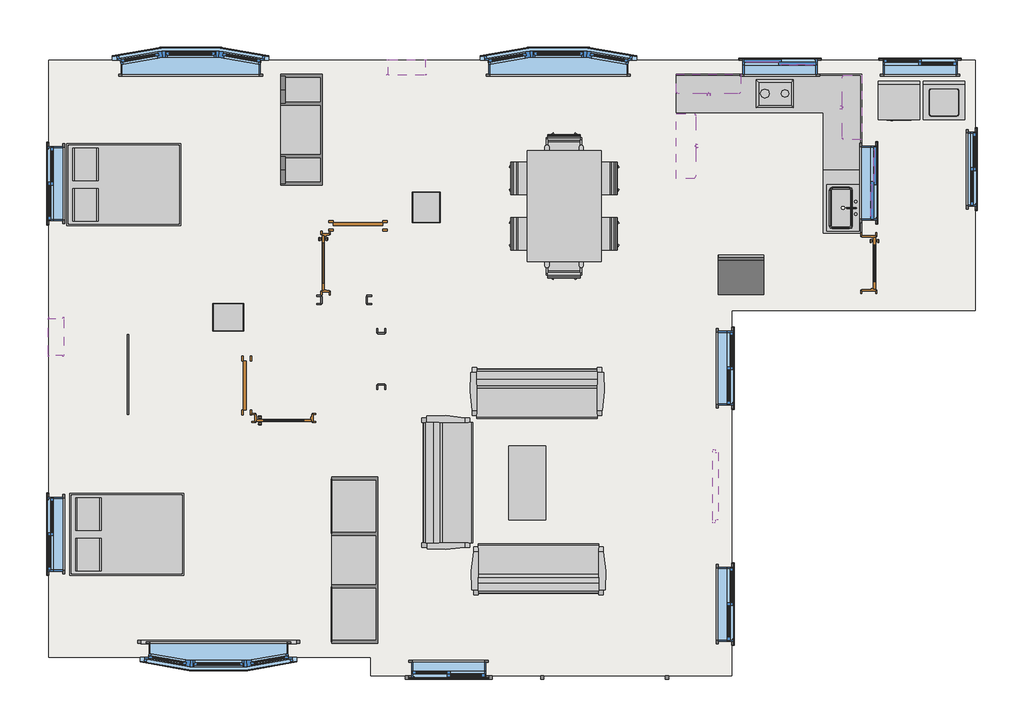
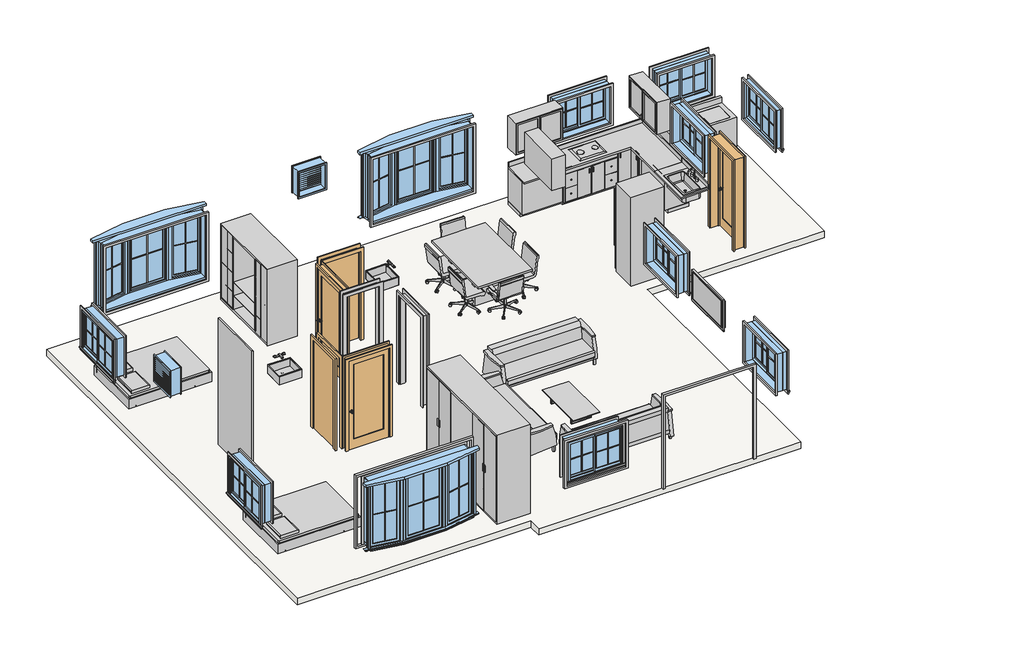
# One storey, incomplete: 54 proxies, 27 furniture elements, 14 windows, 5 doors, 3 flow terminals, 1 plate, 1 slab.
# Revit data of these elements (continued)
# Type "Window-Bay-Casement-10_Degree_Angle : 90\" x 60\" x 6\"" (continued)
#   Exterior Trim = element 406593
#   Interior Trim = Trim-Window-Interior-Flat : Picture Frame
#   Interior Frame Material = Wood - Stained
#   Glass Panel Material = Glass
#   Exterior Frame Material = Clad - White
#   Wall Closure = (empty or 0)
# Type "Window-Louvers : 24\" x 24\""
#   Type Mark = "21"
#   Construction Type Id = "GSP4R"
#   Assembly Code = "B20"
#   Analytic Construction = "1/8 in Pilkington single glazing"
#   Visual Light Transmittance = 0.9
#   Thermal Resistance (R) = 1.53941 (h·ft²·°F)/BTU
#   Solar Heat Gain Coefficient = 0.78
#   Max Height = 1' - 11.74264"
#   Height = 2' - 0"
#   Heat Transfer Coefficient (U) = 0.6496 BTU/(h·ft²·°F)
#   Blade Width [instance default] = 1' - 10 1/2"
#   Blade Vertical Thickness = 0' - 0.35355"
#   Blade Thickness = 0' - 0 1/4"
#   Blade Spacing = 0' - 1 1/2"
#   Blade Height = 0' - 1.85355"
#   Blade Depth = 0' - 3"
#   Blade Angle = 45.00°
#   Default Sill Height = 3' - 0"
#   Trim Projection_Exterior = 0' - 0 1/2"
#   Trim Projection_Interior = 0' - 0 1/2"
#   Trim Width_Exterior = 0' - 1 1/2"
#   Trim Width_Interior = 0' - 1 1/2"
#   Width = 2' - 0"
#   Max Blade Count = 12
#   Define Thermal Properties by = 1
#   Blade Count = 12
#   Frame Material = Birch
#   Louver Material = Birch
#   Trim Exterior Material = Birch
#   Trim Interior Material = Birch
#   Wall Closure = (empty or 0)
# Type "Window-Sliding-Double : 48\" x 36\""
#   Type Mark = "20"
#   Fire Rating = "0.5h"
#   Assembly Code = "B2020100"
#   Analytic Construction = "Double glazing - domestic"
#   Window Inset [instance default] = 0' - 0"
#   Wall Thickness [instance default] = 0' - 6"
#   Visual Light Transmittance = 0.81
#   Thermal Resistance (R) = 1.8146 (h·ft²·°F)/BTU
#   Solar Heat Gain Coefficient = 0.76
#   Muntin Width = 1' - 8 5/8"
#   Muntin Height = 2' - 6 1/4"
#   Interior Wall Closure [instance default] = 0' - 2 3/4"
#   Heat Transfer Coefficient (U) = 0.5511 BTU/(h·ft²·°F)
#   Frame Extension [instance default] = 0' - 0 1/4"
#   Exterior Wall Closure [instance default] = 0' - 1 1/4"
#   Rough Width = 4' - 0 1/2"
#   Rough Height = 3' - 0 1/2"
#   Height = 3' - 0"
#   Extension Jamb [instance default] = 0' - 2 3/4"
#   Default Sill Height = 3' - 0"
#   Width = 4' - 0"
#   Interior Trim Visibility [instance default] = yes
#   Indicator Visibility [instance default] = yes
#   Exterior Trim Visibility [instance default] = yes
#   Muntin Visibility = yes
#   Extension Jamb Visibility [instance default] = yes
#   Muntin Pattern = Muntin Pattern_2x2 : Muntin Pattern_2x2
#   Interior Trim Material = Wood - Stained
#   Interior Trim = Trim-Window-Interior-Flat : Picture Frame
#   Interior Frame Material = Wood - Stained
#   Glass Panel Material = Glass
#   Exterior Trim Material = Clad - White
#   Exterior Trim = Trim-Window-Exterior-Flat : with Sill
#   Exterior Frame Material = Clad - White
#   Wall Closure = (empty or 0)
# Element 1 (IfcBuildingElementProxy, "Cook Top-2 Unit : 12\" x 18\" 2")
#   Phase Created = New Construction
#   Materials on its faces: "Metal - Steel, Polished", "Metal - Chrome"
# Element 2 (IfcBuildingElementProxy, "Dryer : 27\" x 25\" x 35\"")
#   Phase Created = New Construction
#   Materials on its faces: "Metal - Paint Finish - Ivory,Glossy"
# Elements 3, 4, 5 (IfcBuildingElementProxy, "Muntin Pattern_2x2 : Muntin Pattern_2x2")
#   Width = 2' - 3.57789"
#   Height = 4' - 6 1/2"
#   Interior Material = Wood - Stained
#   Exterior Material = Clad - White
#   Phase Created = New Construction
#   Materials on its faces: "Clad - White", "Wood - Stained"
# Elements 6, 7, 8, 9, 10, 11 (IfcBuildingElementProxy, "Muntin Pattern_2x2 : Muntin Pattern_2x2")
#   Width = 1' - 7.85416"
#   Height = 4' - 6 1/2"
#   Interior Material = Wood - Stained
#   Exterior Material = Clad - White
#   Phase Created = New Construction
#   Materials on its faces: "Clad - White", "Wood - Stained"
# Elements 12, 13, 14, 15, 16, 17, 18, 19, 20, 21, 22, 23, 24, 25, 26, 27, 28, 29 (IfcBuildingElementProxy, "Muntin Pattern_2x2 : Muntin Pattern_2x2")
#   Width = 1' - 8 5/8"
#   Height = 2' - 6 1/4"
#   Interior Material = Wood - Stained
#   Exterior Material = Clad - White
#   Phase Created = New Construction
#   Materials on its faces: "Clad - White", "Wood - Stained"
# Element 30 (IfcBuildingElementProxy, "Passage Opening-Cased : 30\" x 84\"")
#   Phase Created = New Construction
#   Materials on its faces: "Door - Frame"
# Element 31 (IfcBuildingElementProxy, "Passage Opening-Cased : 34\" x 84\"")
#   Phase Created = New Construction
#   Materials on its faces: "Door - Frame"
# Element 32 (IfcBuildingElementProxy, "Refrigerator-Built-in : 30\" x 24\" LH")
#   Phase Created = New Construction
#   Materials on its faces: "Metal - Paint Finish - Ivory,Glossy", "Metal - Chrome"
# Elements 33, 34, 35, 36, 37, 38, 39, 40, 41 (IfcBuildingElementProxy, "Trim-Window-Exterior-Flat : with Sill")
#   Opening Width = 4' - 0"
#   Opening Height = 3' - 0"
#   Trim Material = Clad - White
#   Phase Created = New Construction
#   Materials on its faces: "Clad - White"
# Elements 42, 43, 44 (IfcBuildingElementProxy, "Trim-Window-Interior-Flat : Picture Frame")
#   Opening Width = 7' - 6"
#   Opening Height = 5' - 2"
#   Trim Material = Wood - Stained
#   Phase Created = New Construction
#   Materials on its faces: "Wood - Stained"
# Elements 45, 46, 47, 48, 49, 50, 51, 52, 53 (IfcBuildingElementProxy, "Trim-Window-Interior-Flat : Picture Frame")
#   Opening Width = 4' - 0"
#   Opening Height = 3' - 0"
#   Trim Material = Wood - Stained
#   Phase Created = New Construction
#   Materials on its faces: "Wood - Stained"
# Element 54 (IfcBuildingElementProxy, "Washer : 27\" x 25\" x 35\"")
#   Phase Created = New Construction
#   Materials on its faces: "Metal - Paint Finish - Ivory,Matte"
# Element 55 (IfcDoor, "Door-Interior-Single-1_Panel-Wood : 34\" x 84\"")
#   Swing Angle = 90.00°
#   Phase Created = New Construction
#   Materials on its faces: "Cherry", "Aluminum"
# Elements 56, 57 (IfcDoor, "Door-Interior-Single-1_Panel-Wood : 36\" x 84\"")
#   Swing Angle = 90.00°
#   Phase Created = New Construction
#   Materials on its faces: "Cherry", "Aluminum"
# Elements 58, 59 (IfcDoor, "Single-Flush : 32\" x 84\"")
#   Phase Created = New Construction
#   Materials on its faces: "Door - Frame", "Door - Panel"
# Element 60 (IfcFlowTerminal, "Sink - Work : 20\"x18\"")
#   Mark = "1"
#   Flow Pressure = 8.00 psi
#   Phase Created = New Construction
# Element 61 (IfcFlowTerminal, "Sink - Work : 20\"x18\"")
#   Mark = "2"
#   Flow Pressure = 8.00 psi
#   Phase Created = New Construction
# Element 62 (IfcFlowTerminal, "Sink Kitchen-Single : 30\" x 21\"")
#   Mark = "5"
#   Phase Created = New Construction
#   Materials on its faces: "Steel, Polished"
# Element 63 (IfcFurniture, "48\" 2")
#   Phase Created = New Construction
#   Materials on its faces: "Cabinets", "Cabinets - Handles"
# Elements 64, 65 (IfcFurniture, "Base Cabinet-Combo01 : 30\" 2")
#   Phase Created = New Construction
#   Materials on its faces: "Cabinet"
# Element 66 (IfcFurniture, "Base Cabinet-Corner Unit-Square : 36\" 2")
#   Phase Created = New Construction
#   Materials on its faces: "Cabinets", "Cabinets - Handles"
# Elements 67, 68 (IfcFurniture, "Bed-Box : Double 53\" x 74\"")
#   Phase Created = New Construction
#   Materials on its faces: "Birch", "Linen, White"
# Element 69 (IfcFurniture, "Casework 2 : Casework 2")
#   Phase Created = New Construction
#   Materials on its faces: "Wood Planks"
# Element 70 (IfcFurniture, "Casework 3 : Casework 3")
#   Phase Created = New Construction
# Elements 71, 72, 73, 74 (IfcFurniture, "Chair-Task : Chair-Task")
#   Phase Created = New Construction
#   Materials on its faces: "Plastic - Black", "Textile - Slate Blue"
# Elements 75, 76 (IfcFurniture, "Chair-Task Arms : Chair-Task Arms")
#   Phase Created = New Construction
#   Materials on its faces: "Plastic - Black", "Textile - Slate Blue"
# Element 77 (IfcFurniture, "Counter Top w Sink Hole : 24\" Depth")
#   Sink Opening Width = 2' - 3"
#   Sink Opening Depth = 1' - 3"
#   Sink Location To Wall = 0' - 6"
#   Sink Location = 2' - 0 5/8"
#   Length = 3' - 5"
#   Phase Created = New Construction
#   Materials on its faces: "Counter Top"
# Element 78 (IfcFurniture, "Counter Top-L Shaped : 24\" Depth")
#   Length - Leg 2 = 10' - 0"
#   Length - Leg 1 = 5' - 2"
#   Phase Created = New Construction
#   Materials on its faces: "Counter Top"
# Element 79 (IfcFurniture, "Entertainment Center.0001 : 72\" x 72\" x 24\"")
#   Phase Created = New Construction
#   Materials on its faces: "Steel, Chrome Plated", "Glass - Clear, Grey"
# Element 80 (IfcFurniture, "Entertainment Center.0001 : 96\" x 84\" x 30\"")
#   Phase Created = New Construction
#   Materials on its faces: "Laminate, Ivory, Matte", "Steel, Chrome Plated", "Glass - Clear, Grey"
# Elements 81, 82, 83 (IfcFurniture, "Sofa-Pensi : 84\"")
#   Phase Created = New Construction
#   Materials on its faces: "Cherry", "Linen, Beige", "Steel, Chrome Plated"
# Element 84 (IfcFurniture, "Table-Coffee Rectangular : 48\" x 24\"")
#   Phase Created = New Construction
#   Materials on its faces: "Metal - Chrome", "Laminate - Ivory,Matte"
# Element 85 (IfcFurniture, "Table-Conference2 w Chairs : 48\" x 144\" 2")
#   Phase Created = New Construction
#   Materials on its faces: "Wood - Cherry"
# Element 86 (IfcFurniture, "Television-Plasma : 50\"")
#   Phase Created = New Construction
#   Materials on its faces: "Plastic - Gray", "Glass"
# Elements 87, 88, 89 (IfcFurniture, "Upper Cabinet-Double Door w Glass-Wall : 42\"")
#   Phase Created = New Construction
#   Materials on its faces: "Cabinets", "Cabinets - Handles", "Glass"
# Element 90 (IfcPlate, "System Panel : Glazed")
#   Phase Created = New Construction
#   Materials on its faces: "Glass"
# Element 91 (IfcSlab, "Generic - 6\"")
#   Height Offset From Level = 0' - 0"
#   Phase Created = New Construction
#   Materials on its faces: "Concrete, Cast-in-Place gray"
# Element 92 (IfcWindow, "Window-Bay-Casement-10_Degree_Angle : 90\" x 60\" x 6\"")
#   Mark = "1"
#   Interior Trim Visibility = yes
#   Exterior Trim Visibility = yes
#   Phase Created = New Construction
#   Materials on its faces: "Clad - White", "Wood - Stained", "Glass"
# Element 93 (IfcWindow, "Window-Bay-Casement-10_Degree_Angle : 90\" x 60\" x 6\"")
#   Mark = "2"
#   Interior Trim Visibility = yes
#   Exterior Trim Visibility = yes
#   Phase Created = New Construction
#   Materials on its faces: "Clad - White", "Wood - Stained", "Glass"
# Element 94 (IfcWindow, "Window-Bay-Casement-10_Degree_Angle : 90\" x 60\" x 6\"")
#   Mark = "3"
#   Interior Trim Visibility = yes
#   Exterior Trim Visibility = yes
#   Phase Created = New Construction
#   Materials on its faces: "Clad - White", "Wood - Stained", "Glass"
# Element 95 (IfcWindow, "Window-Louvers : 24\" x 24\"")
#   Mark = "12"
#   Blade Width = 1' - 10 1/2"
#   Phase Created = New Construction
#   Materials on its faces: "Birch"
# Element 96 (IfcWindow, "Window-Louvers : 24\" x 24\"")
#   Mark = "13"
#   Blade Width = 1' - 10 1/2"
#   Phase Created = New Construction
#   Materials on its faces: "Birch"
# Element 97 (IfcWindow, "Window-Sliding-Double : 48\" x 36\"")
#   Mark = "5"
#   Window Inset = 0' - 0"
#   Interior Wall Closure = 0' - 2 3/4"
#   Frame Extension = 0' - 0 1/4"
#   Exterior Wall Closure = 0' - 1 1/4"
#   Interior Trim Visibility = yes
#   Indicator Visibility = yes
#   Exterior Trim Visibility = yes
#   Phase Created = New Construction
#   Materials on its faces: "Wood - Stained", "Glass", "Clad - White"
# Element 98 (IfcWindow, "Window-Sliding-Double : 48\" x 36\"")
#   Mark = "6"
#   Window Inset = 0' - 0"
#   Interior Wall Closure = 0' - 2 3/4"
#   Frame Extension = 0' - 0 1/4"
#   Exterior Wall Closure = 0' - 1 1/4"
#   Interior Trim Visibility = yes
#   Indicator Visibility = yes
#   Exterior Trim Visibility = yes
#   Phase Created = New Construction
#   Materials on its faces: "Wood - Stained", "Glass", "Clad - White"
# Element 99 (IfcWindow, "Window-Sliding-Double : 48\" x 36\"")
#   Mark = "7"
#   Window Inset = 0' - 0"
#   Interior Wall Closure = 0' - 2 3/4"
#   Frame Extension = 0' - 0 1/4"
#   Exterior Wall Closure = 0' - 1 1/4"
#   Interior Trim Visibility = yes
#   Indicator Visibility = yes
#   Exterior Trim Visibility = yes
#   Phase Created = New Construction
#   Materials on its faces: "Wood - Stained", "Glass", "Clad - White"
# Element 100 (IfcWindow, "Window-Sliding-Double : 48\" x 36\"")
#   Mark = "8"
#   Window Inset = 0' - 0"
#   Interior Wall Closure = 0' - 2 3/4"
#   Frame Extension = 0' - 0 1/4"
#   Exterior Wall Closure = 0' - 1 1/4"
#   Interior Trim Visibility = yes
#   Indicator Visibility = yes
#   Exterior Trim Visibility = yes
#   Phase Created = New Construction
#   Materials on its faces: "Wood - Stained", "Glass", "Clad - White"
# Element 101 (IfcWindow, "Window-Sliding-Double : 48\" x 36\"")
#   Mark = "9"
#   Window Inset = 0' - 0"
#   Interior Wall Closure = 0' - 2 3/4"
#   Frame Extension = 0' - 0 1/4"
#   Exterior Wall Closure = 0' - 1 1/4"
#   Interior Trim Visibility = yes
#   Indicator Visibility = yes
#   Exterior Trim Visibility = yes
#   Phase Created = New Construction
#   Materials on its faces: "Wood - Stained", "Glass", "Clad - White"
# Element 102 (IfcWindow, "Window-Sliding-Double : 48\" x 36\"")
#   Mark = "10"
#   Window Inset = 0' - 0"
#   Interior Wall Closure = 0' - 2 3/4"
#   Frame Extension = 0' - 0 1/4"
#   Exterior Wall Closure = 0' - 1 1/4"
#   Interior Trim Visibility = yes
#   Indicator Visibility = yes
#   Exterior Trim Visibility = yes
#   Phase Created = New Construction
#   Materials on its faces: "Wood - Stained", "Glass", "Clad - White"
# Element 103 (IfcWindow, "Window-Sliding-Double : 48\" x 36\"")
#   Mark = "11"
#   Window Inset = 0' - 0"
#   Interior Wall Closure = 0' - 2 3/4"
#   Frame Extension = 0' - 0 1/4"
#   Exterior Wall Closure = 0' - 1 1/4"
#   Interior Trim Visibility = yes
#   Indicator Visibility = yes
#   Exterior Trim Visibility = yes
#   Phase Created = New Construction
#   Materials on its faces: "Wood - Stained", "Glass", "Clad - White"
# Element 104 (IfcWindow, "Window-Sliding-Double : 48\" x 36\"")
#   Mark = "15"
#   Window Inset = 0' - 0"
#   Interior Wall Closure = 0' - 2 3/4"
#   Frame Extension = 0' - 0 1/4"
#   Exterior Wall Closure = 0' - 1 1/4"
#   Interior Trim Visibility = yes
#   Indicator Visibility = yes
#   Exterior Trim Visibility = yes
#   Phase Created = New Construction
#   Materials on its faces: "Wood - Stained", "Glass", "Clad - White"
# Element 105 (IfcWindow, "Window-Sliding-Double : 48\" x 36\"")
#   Mark = "14"
#   Window Inset = 0' - 0"
#   Interior Wall Closure = 0' - 2 3/4"
#   Frame Extension = 0' - 0 1/4"
#   Exterior Wall Closure = 0' - 1 1/4"
#   Interior Trim Visibility = yes
#   Indicator Visibility = yes
#   Exterior Trim Visibility = yes
#   Phase Created = New Construction
#   Materials on its faces: "Wood - Stained", "Glass", "Clad - White"
# Materials
#   "Metal - Chrome": colour RGB 57 57 57, transparency 0
#   "Metal - Steel, Polished": colour RGB 57 57 57, transparency 0
#   "Metal - Paint Finish - Ivory,Glossy": colour RGB 247 247 239, transparency 0
#   "Door - Frame": colour RGB 118 70 51, transparency 0, Cost = 0
#   "Metal - Paint Finish - Ivory,Matte": colour RGB 247 247 239, transparency 0
#   "Cherry": class "Wood", colour RGB 226 177 128, transparency 0, Description = "Prunus Serotina", Cost = 0
#   "Aluminum": class "Metal", colour RGB 247 247 247, transparency 0, Description = "Aluminum 6061", Cost = 0
#   "Door - Panel": class "Wood", colour RGB 210 159 95, transparency 0, Cost = 0
#   "Steel, Polished": class "Metal", colour RGB 57 57 57, transparency 0, Description = "Polished steel", Cost = 0
#   "Cabinets - Handles": colour RGB 57 57 57, transparency 0
#   "Cabinets": colour RGB 249 249 249, transparency 0
#   "Birch": class "Wood", colour RGB 224 178 126, transparency 0, Description = "Betula Alleghaniensis", Cost = 0
#   "Linen, White": class "Textile", colour RGB 247 247 239, transparency 0, Description = "Linen, white", Cost = 0
#   "Plastic - Black": colour RGB 0 0 0, transparency 0
#   "Textile - Slate Blue": colour RGB 98 102 118, transparency 0
#   "Laminate, Ivory, Matte": class "Plastic", colour RGB 247 247 239, transparency 0, Description = "Plastic Laminate - Ivory, Matte", Cost = 0
#   "Linen, Beige": class "Textile", colour RGB 249 239 230, transparency 0, Description = "Linen, beige", Cost = 0
#   "Steel, Chrome Plated": class "Metal", colour RGB 17 17 17, transparency 0, Description = "Chromiuim plated steel", Cost = 0
#   "Laminate - Ivory,Matte": colour RGB 247 247 239, transparency 0
#   "Wood - Cherry": colour RGB 151 75 0, transparency 0
#   "Plastic - Gray": colour RGB 134 134 134, transparency 0
#   "Glass": class "Glass", colour RGB 0 128 192, transparency 0.75, Description = "Soda Lime Glass", Cost = 0
#   "Concrete, Cast-in-Place gray": class "Concrete", colour RGB 192 192 192, transparency 0, Description = "Cast-in-place concrete", Cost = 0
#   "Wood - Stained": class "Wood", colour RGB 224 178 126, transparency 0, Cost = 0
#   "Clad - White": class "Wood", colour RGB 242 242 238, transparency 0, Cost = 0
#   "Cabinet": colour RGB 204 122 2, transparency 0
#   "Wood Planks": class "Wood", colour RGB 193 160 115, transparency 0, Description = "Physical material.", Cost = 0
#   "Counter Top": class "Wood", colour RGB 226 177 128, transparency 0
#   "Glass - Clear, Grey": class "Glass", colour RGB 252 255 255, transparency 0.64
